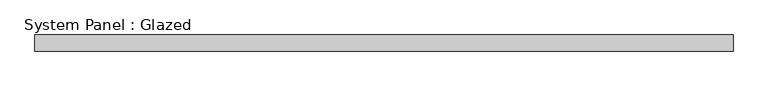
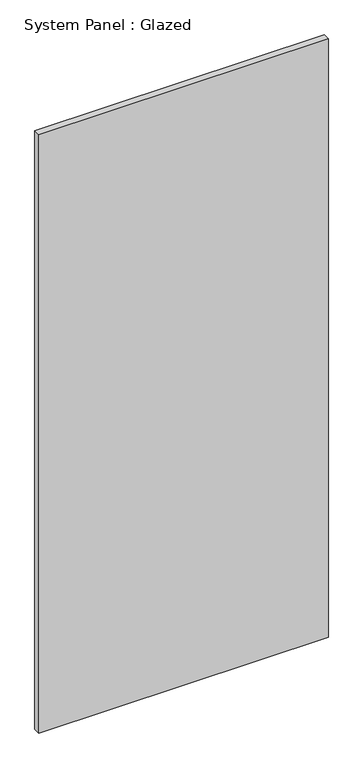
"""IFC4 building model written with IfcOpenShell, lengths in millimetres: plate geometry, System Panel : Glazed."""

from ifc_helpers import new_model, si_unit, origin, origin_with_axes, place, context, project, spatial, polyline, outline, extrude, source, transform, mapped, element, save


def system_panel_glazed_2e981f09(model_context):
    return source(origin(), model_context, "Body", "SweptSolid", [
        extrude(outline(polyline([(536.5750001, 19.05), (-536.5750001, 19.05), (-536.5750001, 44.45), (536.5750001, 44.45), (536.5750001, 19.05)])), origin_with_axes(), (0.0, 0.0, 1.0), 2343.15),
    ])


if __name__ == "__main__":
    model = new_model("IFC4")
    model_context = context("Model", 3, world=origin())
    ifc_project = project(units=[si_unit("LENGTHUNIT", "METRE", prefix="MILLI")], contexts=[model_context])
    site = spatial("IfcSite", under=ifc_project)
    building = spatial("IfcBuilding", under=site)
    placement = place(None, origin())
    system_panel_glazed_shape = system_panel_glazed_2e981f09(model_context)
    element("IfcPlate", 1, ObjectType="System Panel : Glazed", at=placement, inside=building, context=model_context, shape_type="MappedRepresentation", body=[
        mapped(system_panel_glazed_shape, transform((0.0, 0.0, 0.0), x_axis=(1.0, 0.0, 0.0), y_axis=(0.0, 1.0, 0.0), z_axis=(0.0, 0.0, 1.0))),
    ])
    save(model, "model.ifc")

# Revit data of these elements
# Type "System Panel : Glazed"
#   Construction Type Id = "GSP4R"
#   Analytic Construction = "1/8 in Pilkington single glazing"
#   Visual Light Transmittance = 0.9
#   Solar Heat Gain Coefficient = 0.86
#   Heat Transfer Coefficient (U) = 1.18115 BTU/(h·ft²·°F)
#   Define Thermal Properties by = 1
# Element 1 (IfcPlate, "System Panel : Glazed")
#   Materials on its faces: "glass panel 223"
# Materials
#   "glass panel 223": class "Generic", colour RGB 120 120 120, transparency 0, Cost = 0
